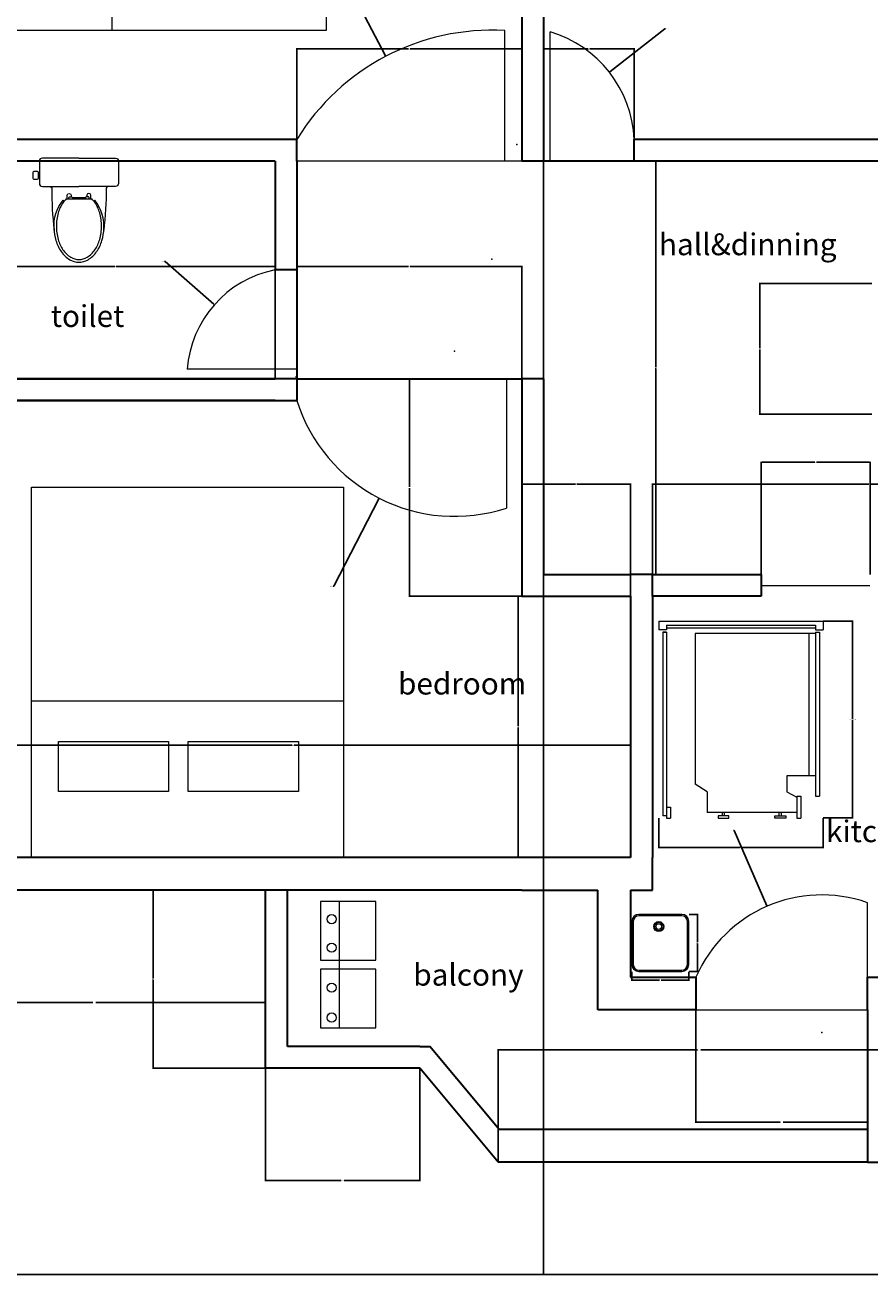
# Model space of a CAD drawing. Units: inches. Extents: x 177 to 785, y -381 to 206.
# Tile 2 of 5: x 296 to 529, y -381 to -37. Entities that reach past the tile are written whole.
import ezdxf

# ---------------------------------------------------------------- set-up
doc = ezdxf.new("R2010")
doc.units = ezdxf.units.IN
doc.header["$MEASUREMENT"] = 0
for name, color, linetype, lineweight in [('A-ANNO-DIMS', 2, 'Continuous', 18), ('A-AREA-IDEN', 7, 'Continuous', 20), ('A-DOOR', 4, 'Continuous', 18), ('A-FLOR-FIXT', 8, 'Continuous', 18), ('A-FURN', 2, 'Continuous', 18), ('A-WALL', 7, 'Continuous', 35), ('equipments', 2, 'Continuous', 18), ('WC-Detail_dwgmodels.com', 9, 'Continuous', 13), ('WC-Outline_dwgmodels.com', 8, 'Continuous', 18)]:
    doc.layers.add(name, color=color, linetype=linetype, lineweight=lineweight)
doc.styles.get("Standard").update_dxf_attribs({"font": 'arial.ttf'})
doc.dimstyles.get("Standard").update_dxf_attribs({"dimtxt": 0.18, "dimasz": 0.18, "dimexe": 0.18, "dimexo": 0.0625, "dimgap": 0.09, "dimtad": 0, "dimtih": 1, "dimtoh": 1, "dimdec": 4, "dimzin": 0, "dimdsep": 46, "dimtxsty": 'Standard', "dimcen": 0.09, "dimadec": 0, "dimazin": 0, "dimtfac": 1, "dimtdec": 4, "dimtofl": 0, "dimtmove": 0, "dimatfit": 3, "dimfxl": 1, "dimtolj": 1, "dimtzin": 0, "dimarcsym": 0})

# ---------------------------------------------------------------- blocks, each defined once
blk = doc.blocks.new('fr1')
at = {"color": 0, "linetype": 'ByBlock'}
for p, q in [((90.8, 438.2), (-210.3, 438.2)), ((-259.7, 390.1), (-259.7, 86.3)), ((-249.7, 390.1), (-249.7, 86.5)), ((90.8, 428.2), (-210.3, 428.2)), ((130.2, 86.5), (130.2, 390.1)), ((140.2, 87.7), (140.2, 390.1)), ((-210.3, 48.2), (90.8, 48.2)), ((-210.3, 38.2), (90.8, 38.2))]:
    blk.add_line(p, q, dxfattribs=at)
for radius in [35, 30, 20]:
    blk.add_circle((-70.8, 353.2), radius)
for centre, radius, start, end in [((-210.3, 388.7), 49.5, 90, 178.38137), ((90.8, 388.7), 49.5, 1.61863, 90), ((-210.3, 388.7), 39.5, 90, 178.38137), ((90.8, 388.7), 39.5, 1.61863, 90), ((-210.3, 87.7), 49.5, 181.61863, 270), ((-210.3, 87.7), 39.5, 181.61863, 270), ((90.8, 87.7), 39.5, 270, 358.38137), ((90.8, 87.7), 49.5, 270, 358.38137)]:
    blk.add_arc(centre, radius, start, end)
at = {"color": 0, "linetype": 'ByBlock', "extrusion": (0, 0, -1)}
blk.add_ellipse((90.8, 87.7), major_axis=(49.5, 0), ratio=1, start_param=0, end_param=0.02825, dxfattribs=at)
blk = doc.blocks.new('dishwasher_smegsta945s')
for p, q in [((0, 90), (75, 90)), ((0, 90), (0, 86)), ((3.5, 86), (0, 86)), ((3.5, 88.1), (71.5, 88.1)), ((3.5, 88.1), (3.5, 86)), ((3.5, 87), (71.5, 87)), ((71.5, 88.1), (71.5, 86)), ((71.5, 86), (75, 86)), ((75, 90), (75, 86)), ((1.7, 85), (1.7, 1)), ((3.5, 85), (1.7, 85)), ((1.7, 85), (3.5, 85)), ((3.5, 85), (3.5, 0)), ((71.5, 84.3), (16.5, 84.3)), ((16.5, 84.3), (16.5, 15.5)), ((68.5, 84.3), (68.5, 19.3)), ((71.5, 85), (71.5, 10)), ((71.5, 85), (73.3, 85)), ((71.5, 85), (73.3, 85)), ((73.3, 85), (73.3, 10)), ((71.5, 19.3), (58.5, 19.3)), ((58.5, 19.3), (58.5, 12)), ((22, 12), (16.5, 15.5)), ((22, 12), (22, 2.5)), ((58.5, 12), (63, 9.5)), ((63, 10), (64.8, 10)), ((63, 10), (63, 0)), ((64.8, 10), (64.8, 0)), ((71.5, 10), (73.3, 10)), ((3.5, 1), (1.7, 1)), ((3.5, 5), (5.3, 5)), ((5.3, 5), (5.3, 0)), ((63, 2.5), (22, 2.5)), ((29, 1), (29, 2.5)), ((30, 1), (30, 2.5)), ((55, 1), (55, 2.5)), ((56, 1), (56, 2.5)), ((63, 0), (64.8, 0)), ((3.5, 0), (5.3, 0))]:
    blk.add_line(p, q)
for points in [[(27, 0), (32, 0), (32, 1), (27, 1)], [(58, 0), (53, 0), (53, 1), (58, 1)]]:
    blk.add_lwpolyline(points, close=True)
blk = doc.blocks.new('BED-DOUBLE')
blk.add_line((58.96, 86.04), (58.96, 0))
for points in [[(0, 86.04), (102.05, 86.04), (102.05, 0), (0, 0)], [(70.1, 73.56), (83.84, 73.56), (83.84, 43.2), (70.1, 43.2)], [(70.1, 37.79), (83.84, 37.79), (83.84, 7.42), (70.1, 7.42)]]:
    blk.add_lwpolyline(points, close=True)
blk = doc.blocks.new('WC-PAN-AND-SEAT')
for points in [[(0, 20.91, -0.279901), (0.43, 20.4, 0.030761), (1.12, 8.8, 16.522544)], [(15.88, 20.91, 0.279901), (15.45, 20.4, -0.030761), (14.76, 8.8, -16.522544)], [(1.72, 9.92, 0.068564), (2.22, 6.28, 0.080689), (3.54, 3.43, 0.107047), (5.7, 1.38, 0.137952), (7.94, 0.75, 0.137952), (10.18, 1.38, 0.107047), (12.34, 3.43, 0.080689), (13.66, 6.28, 0.068564), (14.16, 9.92, 0.068564), (13.66, 13.57, 0.080689), (12.34, 16.41, 0.049741), (11.45, 17.48, 0.137952)], [(4.44, 17.48, 0.049741), (3.54, 16.41, 0.080689), (2.22, 13.57, 0.068564), (1.72, 9.92, 0.068564)], [(1.08, 9.29, -0.186192), (3.55, 17.08), (3.86, 16.84)], [(14.76, 8.8, 0.197511), (12.33, 17.08), (12.02, 16.84)], [(1.07, 9.29, 0.059006), (1.61, 5.99, 0.081908), (3.07, 2.91, 0.106902), (5.45, 0.69, 0.135271), (7.94, 0, 0.135271)], [(1.12, 8.8, -0.010918), (1.08, 9.29)], [(7.94, 0, 0.135271), (10.44, 0.69, 0.106902), (12.81, 2.91, 0.081908), (14.28, 5.99, 0.059006), (14.82, 9.29, 0.070136)]]:
    blk.add_lwpolyline(points, format="xyb")
blk.add_lwpolyline([(4.44, 17.48), (11.45, 17.48)])
blk = doc.blocks.new('*D19')
at = {"layer": 'A-ANNO-DIMS', "color": 0, "lineweight": -2, "transparency": 16777216}
for p, q in [((479.47, -281.84), (481.94, -281.84)), ((481.76, -282.02), (481.76, -289.54)), ((481.76, -297.41), (481.76, -289.9)), ((479.47, -297.59), (481.94, -297.59))]:
    blk.add_line(p, q, dxfattribs=at)
at = {"layer": 'A-ANNO-DIMS', "color": 0, "transparency": 16777216}
for points in [[(481.73, -282.02), (481.79, -282.02), (481.76, -281.84)], [(481.73, -297.41), (481.79, -297.41), (481.76, -297.59)]]:
    blk.add_solid(points, dxfattribs=at)
at = {"layer": 'Defpoints', "color": 0, "transparency": 16777216}
for p in [(479.4, -281.84), (481.76, -281.84), (479.4, -297.59)]:
    blk.add_point(p, dxfattribs=at)
at = {"layer": 'A-ANNO-DIMS', "color": 0, "transparency": 16777216, "insert": (481.76, -289.72), "char_height": 0.18, "attachment_point": 5}
blk.add_mtext('\\A1;SINK 16', dxfattribs=at)
blk = doc.blocks.new('*D20')
at = {"layer": 'A-ANNO-DIMS', "color": 0, "lineweight": -2, "transparency": 16777216}
for p, q in [((463.66, -297.66), (463.66, -300.13)), ((479.4, -297.66), (479.4, -300.13)), ((463.84, -299.95), (471.32, -299.95)), ((479.22, -299.95), (471.74, -299.95))]:
    blk.add_line(p, q, dxfattribs=at)
at = {"layer": 'A-ANNO-DIMS', "color": 0, "transparency": 16777216}
for points in [[(463.84, -299.92), (463.84, -299.98), (463.66, -299.95)], [(479.22, -299.92), (479.22, -299.98), (479.4, -299.95)]]:
    blk.add_solid(points, dxfattribs=at)
at = {"layer": 'Defpoints', "color": 0, "transparency": 16777216}
for p in [(463.66, -297.59), (479.4, -297.59), (479.4, -299.95)]:
    blk.add_point(p, dxfattribs=at)
at = {"layer": 'A-ANNO-DIMS', "color": 0, "transparency": 16777216, "insert": (471.53, -299.95), "char_height": 0.18, "attachment_point": 5}
blk.add_mtext('\\A1;16', dxfattribs=at)
blk = doc.blocks.new('*D21')
at = {"layer": 'A-ANNO-DIMS', "color": 0, "lineweight": -2, "transparency": 16777216}
for p, q in [((516.45, -200.99), (524.71, -200.99)), ((524.53, -201.17), (524.53, -227.94)), ((524.53, -255.08), (524.53, -228.31)), ((516.45, -255.26), (524.71, -255.26))]:
    blk.add_line(p, q, dxfattribs=at)
at = {"layer": 'A-ANNO-DIMS', "color": 0, "transparency": 16777216}
for points in [[(524.5, -201.17), (524.56, -201.17), (524.53, -200.99)], [(524.5, -255.08), (524.56, -255.08), (524.53, -255.26)]]:
    blk.add_solid(points, dxfattribs=at)
at = {"layer": 'Defpoints', "color": 0, "transparency": 16777216}
for p in [(516.39, -200.99), (524.53, -200.99), (516.39, -255.26)]:
    blk.add_point(p, dxfattribs=at)
at = {"layer": 'A-ANNO-DIMS', "color": 0, "transparency": 16777216, "insert": (524.53, -228.12), "char_height": 0.18, "attachment_point": 5}
blk.add_mtext('\\A1;DISHWASHER 54', dxfattribs=at)
blk = doc.blocks.new('*D22')
at = {"layer": 'A-ANNO-DIMS', "color": 0, "lineweight": -2, "transparency": 16777216}
for p, q in [((471.16, -255.32), (471.16, -263.58)), ((516.39, -255.32), (516.39, -263.58)), ((471.34, -263.4), (493.55, -263.4)), ((516.21, -263.4), (494, -263.4))]:
    blk.add_line(p, q, dxfattribs=at)
at = {"layer": 'A-ANNO-DIMS', "color": 0, "transparency": 16777216}
for points in [[(471.34, -263.37), (471.34, -263.43), (471.16, -263.4)], [(516.21, -263.37), (516.21, -263.43), (516.39, -263.4)]]:
    blk.add_solid(points, dxfattribs=at)
at = {"layer": 'Defpoints', "color": 0, "transparency": 16777216}
for p in [(471.16, -255.26), (516.39, -255.26), (516.39, -263.4)]:
    blk.add_point(p, dxfattribs=at)
at = {"layer": 'A-ANNO-DIMS', "color": 0, "transparency": 16777216, "insert": (493.77, -263.4), "char_height": 0.18, "attachment_point": 5}
blk.add_mtext('\\A1;45', dxfattribs=at)
blk = doc.blocks.new('*D23')
at = {"layer": 'A-ANNO-DIMS', "color": 0, "lineweight": -2, "transparency": 16777216}
for p, q in [((754.33, -257.2), (754.33, -381.27)), ((202.33, -275.2), (202.33, -381.27)), ((202.51, -381.09), (478.04, -381.09)), ((754.15, -381.09), (478.62, -381.09))]:
    blk.add_line(p, q, dxfattribs=at)
at = {"layer": 'A-ANNO-DIMS', "color": 0, "transparency": 16777216}
for points in [[(202.51, -381.06), (202.51, -381.12), (202.33, -381.09)], [(754.15, -381.06), (754.15, -381.12), (754.33, -381.09)]]:
    blk.add_solid(points, dxfattribs=at)
at = {"layer": 'Defpoints', "color": 0, "transparency": 16777216}
for p in [(754.33, -257.14), (202.33, -275.14), (754.33, -381.09)]:
    blk.add_point(p, dxfattribs=at)
at = {"layer": 'A-ANNO-DIMS', "color": 0, "transparency": 16777216, "insert": (478.33, -381.09), "char_height": 0.18, "attachment_point": 5}
blk.add_mtext('\\A1;552', dxfattribs=at)
blk = doc.blocks.new('*D33')
at = {"layer": 'A-ANNO-DIMS', "color": 0, "lineweight": -2, "transparency": 16777216}
for p, q in [((607.33, -68.2), (607.33, -381.27)), ((439.33, -74.2), (439.33, -381.27)), ((439.51, -381.09), (523.05, -381.09)), ((607.15, -381.09), (523.61, -381.09))]:
    blk.add_line(p, q, dxfattribs=at)
at = {"layer": 'A-ANNO-DIMS', "color": 0, "transparency": 16777216}
for points in [[(439.51, -381.06), (439.51, -381.12), (439.33, -381.09)], [(607.15, -381.06), (607.15, -381.12), (607.33, -381.09)]]:
    blk.add_solid(points, dxfattribs=at)
at = {"layer": 'Defpoints', "color": 0, "transparency": 16777216}
for p in [(607.33, -68.14), (439.33, -74.14), (607.33, -381.09)]:
    blk.add_point(p, dxfattribs=at)
at = {"layer": 'A-ANNO-DIMS', "color": 0, "transparency": 16777216, "insert": (523.33, -381.09), "char_height": 0.18, "attachment_point": 5}
blk.add_mtext('\\A1;168', dxfattribs=at)
blk = doc.blocks.new('*D41')
at = {"layer": 'A-ANNO-DIMS', "color": 0, "lineweight": -2, "transparency": 16777216}
for p, q in [((277.33, -134.08), (277.33, -103.01)), ((277.51, -103.19), (321.11, -103.19)), ((365.15, -103.19), (321.55, -103.19)), ((365.33, -134.08), (365.33, -103.01))]:
    blk.add_line(p, q, dxfattribs=at)
at = {"layer": 'A-ANNO-DIMS', "color": 0, "transparency": 16777216}
for points in [[(277.51, -103.16), (277.51, -103.22), (277.33, -103.19)], [(365.15, -103.16), (365.15, -103.22), (365.33, -103.19)]]:
    blk.add_solid(points, dxfattribs=at)
at = {"layer": 'Defpoints', "color": 0, "transparency": 16777216}
for p in [(365.33, -103.19), (277.33, -134.14), (365.33, -134.14)]:
    blk.add_point(p, dxfattribs=at)
at = {"layer": 'A-ANNO-DIMS', "color": 0, "transparency": 16777216, "insert": (321.33, -103.19), "char_height": 0.18, "attachment_point": 5}
blk.add_mtext('\\A1;88', dxfattribs=at)
blk = doc.blocks.new('*D45')
at = {"layer": 'A-ANNO-DIMS', "color": 0, "lineweight": -2, "transparency": 16777216}
for p, q in [((277.33, -266.08), (277.33, -235.01)), ((277.51, -235.19), (370.05, -235.19)), ((463.15, -235.19), (370.61, -235.19)), ((463.33, -266.08), (463.33, -235.01))]:
    blk.add_line(p, q, dxfattribs=at)
at = {"layer": 'A-ANNO-DIMS', "color": 0, "transparency": 16777216}
for points in [[(277.51, -235.16), (277.51, -235.22), (277.33, -235.19)], [(463.15, -235.16), (463.15, -235.22), (463.33, -235.19)]]:
    blk.add_solid(points, dxfattribs=at)
at = {"layer": 'Defpoints', "color": 0, "transparency": 16777216}
for p in [(463.33, -235.19), (277.33, -266.14), (463.33, -266.14)]:
    blk.add_point(p, dxfattribs=at)
at = {"layer": 'A-ANNO-DIMS', "color": 0, "transparency": 16777216, "insert": (370.33, -235.19), "char_height": 0.18, "attachment_point": 5}
blk.add_mtext('\\A1;186', dxfattribs=at)
blk = doc.blocks.new('*D46')
at = {"layer": 'A-ANNO-DIMS', "color": 0, "lineweight": -2, "transparency": 16777216}
for p, q in [((433.27, -134.14), (402.2, -134.14)), ((402.38, -134.32), (402.38, -163.96)), ((402.38, -193.96), (402.38, -164.32)), ((433.27, -194.14), (402.2, -194.14))]:
    blk.add_line(p, q, dxfattribs=at)
at = {"layer": 'A-ANNO-DIMS', "color": 0, "transparency": 16777216}
for points in [[(402.35, -134.32), (402.41, -134.32), (402.38, -134.14)], [(402.35, -193.96), (402.41, -193.96), (402.38, -194.14)]]:
    blk.add_solid(points, dxfattribs=at)
at = {"layer": 'Defpoints', "color": 0, "transparency": 16777216}
for p in [(402.38, -134.14), (433.33, -134.14), (433.33, -194.14)]:
    blk.add_point(p, dxfattribs=at)
at = {"layer": 'A-ANNO-DIMS', "color": 0, "transparency": 16777216, "insert": (402.38, -164.14), "char_height": 0.18, "attachment_point": 5}
blk.add_mtext('\\A1;60', dxfattribs=at)
blk = doc.blocks.new('*D47')
at = {"layer": 'A-ANNO-DIMS', "color": 0, "lineweight": -2, "transparency": 16777216}
for p, q in [((463.27, -194.14), (432.2, -194.14)), ((432.38, -194.32), (432.38, -229.96)), ((432.38, -265.96), (432.38, -230.32)), ((463.27, -266.14), (432.2, -266.14))]:
    blk.add_line(p, q, dxfattribs=at)
at = {"layer": 'A-ANNO-DIMS', "color": 0, "transparency": 16777216}
for points in [[(432.35, -194.32), (432.41, -194.32), (432.38, -194.14)], [(432.35, -265.96), (432.41, -265.96), (432.38, -266.14)]]:
    blk.add_solid(points, dxfattribs=at)
at = {"layer": 'Defpoints', "color": 0, "transparency": 16777216}
for p in [(432.38, -194.14), (463.33, -194.14), (463.33, -266.14)]:
    blk.add_point(p, dxfattribs=at)
at = {"layer": 'A-ANNO-DIMS', "color": 0, "transparency": 16777216, "insert": (432.38, -230.14), "char_height": 0.18, "attachment_point": 5}
blk.add_mtext('\\A1;72', dxfattribs=at)
blk = doc.blocks.new('*D48')
at = {"layer": 'A-ANNO-DIMS', "color": 0, "lineweight": -2, "transparency": 16777216}
for p, q in [((433.33, -194.08), (433.33, -163.01)), ((433.51, -163.19), (448.11, -163.19)), ((463.15, -163.19), (448.55, -163.19)), ((463.33, -194.08), (463.33, -163.01))]:
    blk.add_line(p, q, dxfattribs=at)
at = {"layer": 'A-ANNO-DIMS', "color": 0, "transparency": 16777216}
for points in [[(433.51, -163.16), (433.51, -163.22), (433.33, -163.19)], [(463.15, -163.16), (463.15, -163.22), (463.33, -163.19)]]:
    blk.add_solid(points, dxfattribs=at)
at = {"layer": 'Defpoints', "color": 0, "transparency": 16777216}
for p in [(463.33, -163.19), (433.33, -194.14), (463.33, -194.14)]:
    blk.add_point(p, dxfattribs=at)
at = {"layer": 'A-ANNO-DIMS', "color": 0, "transparency": 16777216, "insert": (448.33, -163.19), "char_height": 0.18, "attachment_point": 5}
blk.add_mtext('\\A1;30', dxfattribs=at)
blk = doc.blocks.new('*D49')
at = {"layer": 'A-ANNO-DIMS', "color": 0, "lineweight": -2, "transparency": 16777216}
for p, q in [((469.33, -194.08), (469.33, -163.01)), ((469.51, -163.19), (529.05, -163.19)), ((589.15, -163.19), (529.61, -163.19)), ((589.33, -194.08), (589.33, -163.01))]:
    blk.add_line(p, q, dxfattribs=at)
at = {"layer": 'A-ANNO-DIMS', "color": 0, "transparency": 16777216}
for points in [[(469.51, -163.16), (469.51, -163.22), (469.33, -163.19)], [(589.15, -163.16), (589.15, -163.22), (589.33, -163.19)]]:
    blk.add_solid(points, dxfattribs=at)
at = {"layer": 'Defpoints', "color": 0, "transparency": 16777216}
for p in [(589.33, -163.19), (469.33, -194.14), (589.33, -194.14)]:
    blk.add_point(p, dxfattribs=at)
at = {"layer": 'A-ANNO-DIMS', "color": 0, "transparency": 16777216, "insert": (529.33, -163.19), "char_height": 0.18, "attachment_point": 5}
blk.add_mtext('\\A1;120', dxfattribs=at)
blk = doc.blocks.new('*D54')
at = {"layer": 'A-ANNO-DIMS', "color": 0, "lineweight": -2, "transparency": 16777216}
for p, q in [((439.39, -74.14), (470.46, -74.14)), ((470.28, -74.32), (470.28, -130.96)), ((470.28, -187.96), (470.28, -131.32)), ((439.39, -188.14), (470.46, -188.14))]:
    blk.add_line(p, q, dxfattribs=at)
at = {"layer": 'A-ANNO-DIMS', "color": 0, "transparency": 16777216}
for points in [[(470.25, -74.32), (470.31, -74.32), (470.28, -74.14)], [(470.25, -187.96), (470.31, -187.96), (470.28, -188.14)]]:
    blk.add_solid(points, dxfattribs=at)
at = {"layer": 'Defpoints', "color": 0, "transparency": 16777216}
for p in [(439.33, -74.14), (439.33, -188.14), (470.28, -188.14)]:
    blk.add_point(p, dxfattribs=at)
at = {"layer": 'A-ANNO-DIMS', "color": 0, "transparency": 16777216, "insert": (470.28, -131.14), "char_height": 0.18, "attachment_point": 5}
blk.add_mtext('\\A1;114', dxfattribs=at)
blk = doc.blocks.new('*D56')
at = {"layer": 'A-ANNO-DIMS', "color": 0, "lineweight": -2, "transparency": 16777216}
for p, q in [((362.64, -275.14), (331.57, -275.14)), ((331.75, -275.32), (331.75, -299.53)), ((331.75, -324.1), (331.75, -299.89)), ((362.64, -324.28), (331.57, -324.28))]:
    blk.add_line(p, q, dxfattribs=at)
at = {"layer": 'A-ANNO-DIMS', "color": 0, "transparency": 16777216}
for points in [[(331.72, -275.32), (331.78, -275.32), (331.75, -275.14)], [(331.72, -324.1), (331.78, -324.1), (331.75, -324.28)]]:
    blk.add_solid(points, dxfattribs=at)
at = {"layer": 'Defpoints', "color": 0, "transparency": 16777216}
for p in [(331.75, -275.14), (362.7, -275.14), (362.7, -324.28)]:
    blk.add_point(p, dxfattribs=at)
at = {"layer": 'A-ANNO-DIMS', "color": 0, "transparency": 16777216, "insert": (331.75, -299.71), "char_height": 0.18, "attachment_point": 5}
blk.add_mtext('\\A1;49.14', dxfattribs=at)
blk = doc.blocks.new('*D57')
at = {"layer": 'A-ANNO-DIMS', "color": 0, "lineweight": -2, "transparency": 16777216}
for p, q in [((426.79, -350.08), (426.79, -319.01)), ((426.97, -319.19), (481.74, -319.19)), ((537.43, -319.19), (482.65, -319.19)), ((537.61, -350.08), (537.61, -319.01))]:
    blk.add_line(p, q, dxfattribs=at)
at = {"layer": 'A-ANNO-DIMS', "color": 0, "transparency": 16777216}
for points in [[(426.97, -319.16), (426.97, -319.22), (426.79, -319.19)], [(537.43, -319.16), (537.43, -319.22), (537.61, -319.19)]]:
    blk.add_solid(points, dxfattribs=at)
at = {"layer": 'Defpoints', "color": 0, "transparency": 16777216}
for p in [(537.61, -319.19), (426.79, -350.14), (537.61, -350.14)]:
    blk.add_point(p, dxfattribs=at)
at = {"layer": 'A-ANNO-DIMS', "color": 0, "transparency": 16777216, "insert": (482.2, -319.19), "char_height": 0.18, "attachment_point": 5}
blk.add_mtext('\\A1;110.82', dxfattribs=at)
blk = doc.blocks.new('*D58')
at = {"layer": 'A-ANNO-DIMS', "color": 0, "lineweight": -2, "transparency": 16777216}
for p, q in [((371.33, -74.08), (371.33, -43.01)), ((371.51, -43.19), (402.11, -43.19)), ((433.15, -43.19), (402.55, -43.19)), ((433.33, -74.08), (433.33, -43.01))]:
    blk.add_line(p, q, dxfattribs=at)
at = {"layer": 'A-ANNO-DIMS', "color": 0, "transparency": 16777216}
for points in [[(371.51, -43.16), (371.51, -43.22), (371.33, -43.19)], [(433.15, -43.16), (433.15, -43.22), (433.33, -43.19)]]:
    blk.add_solid(points, dxfattribs=at)
at = {"layer": 'Defpoints', "color": 0, "transparency": 16777216}
for p in [(433.33, -43.19), (371.33, -74.14), (433.33, -74.14)]:
    blk.add_point(p, dxfattribs=at)
at = {"layer": 'A-ANNO-DIMS', "color": 0, "transparency": 16777216, "insert": (402.33, -43.19), "char_height": 0.18, "attachment_point": 5}
blk.add_mtext('\\A1;62', dxfattribs=at)
blk = doc.blocks.new('*D59')
at = {"layer": 'A-ANNO-DIMS', "color": 0, "lineweight": -2, "transparency": 16777216}
for p, q in [((439.33, -74.08), (439.33, -43.01)), ((439.51, -43.19), (451.61, -43.19)), ((464.15, -43.19), (452.05, -43.19)), ((464.33, -74.08), (464.33, -43.01))]:
    blk.add_line(p, q, dxfattribs=at)
at = {"layer": 'A-ANNO-DIMS', "color": 0, "transparency": 16777216}
for points in [[(439.51, -43.16), (439.51, -43.22), (439.33, -43.19)], [(464.15, -43.16), (464.15, -43.22), (464.33, -43.19)]]:
    blk.add_solid(points, dxfattribs=at)
at = {"layer": 'Defpoints', "color": 0, "transparency": 16777216}
for p in [(464.33, -43.19), (439.33, -74.14), (464.33, -74.14)]:
    blk.add_point(p, dxfattribs=at)
at = {"layer": 'A-ANNO-DIMS', "color": 0, "transparency": 16777216, "insert": (451.83, -43.19), "char_height": 0.18, "attachment_point": 5}
blk.add_mtext('\\A1;25', dxfattribs=at)
blk = doc.blocks.new('*D60')
at = {"layer": 'A-ANNO-DIMS', "color": 0, "lineweight": -2, "transparency": 16777216}
for p, q in [((371.33, -134.08), (371.33, -103.01)), ((371.51, -103.19), (402.11, -103.19)), ((433.15, -103.19), (402.55, -103.19)), ((433.33, -134.08), (433.33, -103.01))]:
    blk.add_line(p, q, dxfattribs=at)
at = {"layer": 'A-ANNO-DIMS', "color": 0, "transparency": 16777216}
for points in [[(371.51, -103.16), (371.51, -103.22), (371.33, -103.19)], [(433.15, -103.16), (433.15, -103.22), (433.33, -103.19)]]:
    blk.add_solid(points, dxfattribs=at)
at = {"layer": 'Defpoints', "color": 0, "transparency": 16777216}
for p in [(433.33, -103.19), (371.33, -134.14), (433.33, -134.14)]:
    blk.add_point(p, dxfattribs=at)
at = {"layer": 'A-ANNO-DIMS', "color": 0, "transparency": 16777216, "insert": (402.33, -103.19), "char_height": 0.18, "attachment_point": 5}
blk.add_mtext('\\A1;62', dxfattribs=at)
blk = doc.blocks.new('*D61')
at = {"layer": 'A-ANNO-DIMS', "color": 0, "lineweight": -2, "transparency": 16777216}
for p, q in [((499.33, -188.08), (499.33, -157.01)), ((499.51, -157.19), (514.11, -157.19)), ((529.15, -157.19), (514.55, -157.19)), ((529.33, -188.08), (529.33, -157.01))]:
    blk.add_line(p, q, dxfattribs=at)
at = {"layer": 'A-ANNO-DIMS', "color": 0, "transparency": 16777216}
for points in [[(499.51, -157.16), (499.51, -157.22), (499.33, -157.19)], [(529.15, -157.16), (529.15, -157.22), (529.33, -157.19)]]:
    blk.add_solid(points, dxfattribs=at)
at = {"layer": 'Defpoints', "color": 0, "transparency": 16777216}
for p in [(529.33, -157.19), (499.33, -188.14), (529.33, -188.14)]:
    blk.add_point(p, dxfattribs=at)
at = {"layer": 'A-ANNO-DIMS', "color": 0, "transparency": 16777216, "insert": (514.33, -157.19), "char_height": 0.18, "attachment_point": 5}
blk.add_mtext('\\A1;30', dxfattribs=at)
blk = doc.blocks.new('*D62')
at = {"layer": 'A-ANNO-DIMS', "color": 0, "lineweight": -2, "transparency": 16777216}
for p, q in [((481.33, -308.2), (481.33, -339.27)), ((528.61, -308.2), (528.61, -339.27)), ((481.51, -339.09), (504.57, -339.09)), ((528.43, -339.09), (505.37, -339.09))]:
    blk.add_line(p, q, dxfattribs=at)
at = {"layer": 'A-ANNO-DIMS', "color": 0, "transparency": 16777216}
for points in [[(481.51, -339.06), (481.51, -339.12), (481.33, -339.09)], [(528.43, -339.06), (528.43, -339.12), (528.61, -339.09)]]:
    blk.add_solid(points, dxfattribs=at)
at = {"layer": 'Defpoints', "color": 0, "transparency": 16777216}
for p in [(481.33, -308.14), (528.61, -308.14), (481.33, -339.09)]:
    blk.add_point(p, dxfattribs=at)
at = {"layer": 'A-ANNO-DIMS', "color": 0, "transparency": 16777216, "insert": (504.97, -339.09), "char_height": 0.18, "attachment_point": 5}
blk.add_mtext('\\A1;47.28', dxfattribs=at)
blk = doc.blocks.new('*D65')
at = {"layer": 'A-ANNO-DIMS', "color": 0, "lineweight": -2, "transparency": 16777216}
for p, q in [((268.33, -275.2), (268.33, -306.27)), ((362.7, -275.2), (362.7, -306.27)), ((268.51, -306.09), (315.12, -306.09)), ((362.52, -306.09), (315.91, -306.09))]:
    blk.add_line(p, q, dxfattribs=at)
at = {"layer": 'A-ANNO-DIMS', "color": 0, "transparency": 16777216}
for points in [[(268.51, -306.06), (268.51, -306.12), (268.33, -306.09)], [(362.52, -306.06), (362.52, -306.12), (362.7, -306.09)]]:
    blk.add_solid(points, dxfattribs=at)
at = {"layer": 'Defpoints', "color": 0, "transparency": 16777216}
for p in [(268.33, -275.14), (362.7, -275.14), (268.33, -306.09)]:
    blk.add_point(p, dxfattribs=at)
at = {"layer": 'A-ANNO-DIMS', "color": 0, "transparency": 16777216, "insert": (315.51, -306.09), "char_height": 0.18, "attachment_point": 5}
blk.add_mtext('\\A1;94.37', dxfattribs=at)
blk = doc.blocks.new('*D67')
at = {"layer": 'A-ANNO-DIMS', "color": 0, "lineweight": -2, "transparency": 16777216}
for p, q in [((529.87, -107.85), (498.8, -107.85)), ((498.98, -108.03), (498.98, -125.71)), ((498.98, -143.76), (498.98, -126.07)), ((529.87, -143.94), (498.8, -143.94))]:
    blk.add_line(p, q, dxfattribs=at)
at = {"layer": 'A-ANNO-DIMS', "color": 0, "transparency": 16777216}
for points in [[(498.95, -108.03), (499.01, -108.03), (498.98, -107.85)], [(498.95, -143.76), (499.01, -143.76), (498.98, -143.94)]]:
    blk.add_solid(points, dxfattribs=at)
at = {"layer": 'Defpoints', "color": 0, "transparency": 16777216}
for p in [(498.98, -107.85), (529.93, -107.85), (529.93, -143.94)]:
    blk.add_point(p, dxfattribs=at)
at = {"layer": 'A-ANNO-DIMS', "color": 0, "transparency": 16777216, "insert": (498.98, -125.89), "char_height": 0.18, "attachment_point": 5}
blk.add_mtext('\\A1;36.09', dxfattribs=at)
blk = doc.blocks.new('*D73')
at = {"layer": 'A-ANNO-DIMS', "color": 0, "lineweight": -2, "transparency": 16777216}
for p, q in [((362.7, -324.34), (362.7, -355.41)), ((405.22, -324.34), (405.22, -355.41)), ((362.88, -355.23), (383.56, -355.23)), ((405.04, -355.23), (384.36, -355.23))]:
    blk.add_line(p, q, dxfattribs=at)
at = {"layer": 'A-ANNO-DIMS', "color": 0, "transparency": 16777216}
for points in [[(362.88, -355.2), (362.88, -355.26), (362.7, -355.23)], [(405.04, -355.2), (405.04, -355.26), (405.22, -355.23)]]:
    blk.add_solid(points, dxfattribs=at)
at = {"layer": 'Defpoints', "color": 0, "transparency": 16777216}
for p in [(362.7, -324.28), (405.22, -324.28), (362.7, -355.23)]:
    blk.add_point(p, dxfattribs=at)
at = {"layer": 'A-ANNO-DIMS', "color": 0, "transparency": 16777216, "insert": (383.96, -355.23), "char_height": 0.18, "attachment_point": 5}
blk.add_mtext('\\A1;42.52', dxfattribs=at)
blk = doc.blocks.new('*D74')
at = {"layer": 'A-ANNO-DIMS', "color": 0, "lineweight": -2, "transparency": 16777216}
for p, q in [((378.1, -11.7), (378.28, -11.7)), ((378.28, -11.7), (395.76, -45.08)), ((425.02, -101.14), (425.2, -101.14)), ((425.11, -101.23), (425.11, -101.05))]:
    blk.add_line(p, q, dxfattribs=at)
at = {"layer": 'A-ANNO-DIMS', "color": 0, "transparency": 16777216}
blk.add_solid([(395.78, -45.07), (395.73, -45.1), (395.84, -45.24)], dxfattribs=at)
at = {"layer": 'Defpoints', "color": 0, "transparency": 16777216}
for p in [(395.84, -45.24), (425.11, -101.14)]:
    blk.add_point(p, dxfattribs=at)
at = {"layer": 'A-ANNO-DIMS', "color": 0, "transparency": 16777216, "insert": (377.7, -11.7), "char_height": 0.18, "attachment_point": 5}
blk.add_mtext('\\A1;R63.1', dxfattribs=at)
blk = doc.blocks.new('*D76')
at = {"layer": 'A-ANNO-DIMS', "color": 0, "lineweight": -2, "transparency": 16777216}
for p, q in [((414.7, -126.55), (414.88, -126.55)), ((414.79, -126.64), (414.79, -126.46)), ((381.51, -191.37), (393.91, -167.22)), ((381.33, -191.37), (381.51, -191.37))]:
    blk.add_line(p, q, dxfattribs=at)
at = {"layer": 'A-ANNO-DIMS', "color": 0, "transparency": 16777216}
blk.add_solid([(393.88, -167.21), (393.94, -167.23), (393.99, -167.06)], dxfattribs=at)
at = {"layer": 'Defpoints', "color": 0, "transparency": 16777216}
for p in [(414.79, -126.55), (393.99, -167.06)]:
    blk.add_point(p, dxfattribs=at)
at = {"layer": 'A-ANNO-DIMS', "color": 0, "transparency": 16777216, "insert": (380.85, -191.37), "char_height": 0.18, "attachment_point": 5}
blk.add_mtext('\\A1;R45.54', dxfattribs=at)
blk = doc.blocks.new('*D77')
at = {"layer": 'A-ANNO-DIMS', "color": 0, "lineweight": -2, "transparency": 16777216}
for p, q in [((491.71, -258.74), (491.89, -258.74)), ((491.89, -258.74), (500.87, -279.44)), ((515.95, -314.38), (516.13, -314.38)), ((516.04, -314.47), (516.04, -314.29))]:
    blk.add_line(p, q, dxfattribs=at)
at = {"layer": 'A-ANNO-DIMS', "color": 0, "transparency": 16777216}
blk.add_solid([(500.9, -279.43), (500.85, -279.45), (500.94, -279.61)], dxfattribs=at)
at = {"layer": 'Defpoints', "color": 0, "transparency": 16777216}
for p in [(500.94, -279.61), (516.04, -314.38)]:
    blk.add_point(p, dxfattribs=at)
at = {"layer": 'A-ANNO-DIMS', "color": 0, "transparency": 16777216, "insert": (491.25, -258.74), "char_height": 0.18, "attachment_point": 5}
blk.add_mtext('\\A1;R37.91', dxfattribs=at)
blk = doc.blocks.new('*D78')
at = {"layer": 'A-ANNO-DIMS', "color": 0, "lineweight": -2, "transparency": 16777216}
for p, q in [((472.76, -37.63), (457.61, -49.5)), ((472.94, -37.63), (472.76, -37.63)), ((431.9, -69.57), (432.08, -69.57)), ((431.99, -69.66), (431.99, -69.48))]:
    blk.add_line(p, q, dxfattribs=at)
at = {"layer": 'A-ANNO-DIMS', "color": 0, "transparency": 16777216}
blk.add_solid([(457.59, -49.47), (457.63, -49.52), (457.47, -49.61)], dxfattribs=at)
at = {"layer": 'Defpoints', "color": 0, "transparency": 16777216}
for p in [(457.47, -49.61), (431.99, -69.57)]:
    blk.add_point(p, dxfattribs=at)
at = {"layer": 'A-ANNO-DIMS', "color": 0, "transparency": 16777216, "insert": (473.42, -37.63), "char_height": 0.18, "attachment_point": 5}
blk.add_mtext('\\A1;R32.37', dxfattribs=at)
blk = doc.blocks.new('*D79')
at = {"layer": 'A-ANNO-DIMS', "color": 0, "lineweight": -2, "transparency": 16777216}
for p, q in [((334.87, -101.79), (335.05, -101.79)), ((335.05, -101.79), (348.44, -113.62)), ((371.03, -133.66), (371.21, -133.66)), ((371.12, -133.75), (371.12, -133.57))]:
    blk.add_line(p, q, dxfattribs=at)
at = {"layer": 'A-ANNO-DIMS', "color": 0, "transparency": 16777216}
blk.add_solid([(348.46, -113.6), (348.42, -113.64), (348.57, -113.74)], dxfattribs=at)
at = {"layer": 'Defpoints', "color": 0, "transparency": 16777216}
for p in [(348.57, -113.74), (371.12, -133.66)]:
    blk.add_point(p, dxfattribs=at)
at = {"layer": 'A-ANNO-DIMS', "color": 0, "transparency": 16777216, "insert": (334.32, -101.79), "char_height": 0.18, "attachment_point": 5}
blk.add_mtext('\\A1;R30.087', dxfattribs=at)

msp = doc.modelspace()

# ---------------------------------------------------------------- linework, layer by layer
at = {"layer": 'A-DOOR'}
for p, q in [((428.6202, -74.1401), (428.6202, -38.1401)), ((441.1154, -74.1401), (441.1154, -38.5162)), ((433.3284, -74.1401), (371.3284, -74.1401)), ((371.3284, -131.5482), (341.106, -131.5482)), ((429.0779, -134.1401), (429.0779, -169.7877)), ((499.3284, -191.1401), (529.3284, -191.1401)), ((528.6096, -308.1401), (528.6096, -278.6179)), ((481.3284, -308.1401), (528.6096, -308.1401))]:
    msp.add_line(p, q, dxfattribs=at)
for centre, radius, start, end in [((425.1088, -101.1401), 63.0978, 86.809847, 148.466446), ((431.9914, -69.5736), 32.3699, 2.538191, 73.628307), ((371.1181, -133.6644), 30.0867, 101.094926, 175.966591), ((414.7917, -126.5473), 45.5393, 197.366629, 288.283034), ((516.0372, -314.379), 37.9068, 70.629909, 156.296067)]:
    msp.add_arc(centre, radius, start, end, dxfattribs=at)
at = {"layer": 'A-WALL'}
for p, q in [((433.3284, 93.8599), (433.3284, -38.1401)), ((439.3284, 93.8599), (439.3284, -38.1401)), ((433.3284, -38.1401), (433.3284, -74.1401)), ((439.3284, -38.1401), (439.3284, -74.1401)), ((371.3284, -68.1401), (277.3284, -68.1401)), ((371.3284, -74.1401), (371.3284, -68.1401)), ((495.3305, -68.1401), (464.3295, -68.1401)), ((464.3295, -74.1401), (464.3295, -68.1401)), ((607.3284, -68.1401), (495.3305, -68.1401)), ((365.3284, -74.1401), (277.3284, -74.1401)), ((365.3284, -74.1401), (365.3284, -104.1401)), ((371.3284, -74.1401), (371.3284, -134.1401)), ((495.3305, -74.1401), (433.3284, -74.1401)), ((613.3284, -74.1401), (495.3305, -74.1401)), ((371.3284, -104.1401), (365.3284, -104.1401)), ((365.3284, -134.1401), (277.3284, -134.1401)), ((277.3284, -134.1401), (365.3284, -134.1401)), ((371.3284, -134.1401), (365.3284, -134.1401)), ((371.3284, -134.1401), (433.3284, -134.1401)), ((371.3284, -134.1401), (371.3284, -140.1401)), ((433.3284, -134.1401), (433.3284, -194.1401)), ((433.3284, -134.1401), (433.3284, -194.1401)), ((439.3284, -134.1401), (433.3284, -134.1401)), ((439.3284, -134.1401), (439.3284, -188.1401)), ((365.3284, -140.1401), (277.3284, -140.1401)), ((277.3284, -140.1401), (371.3284, -140.1401)), ((365.3284, -140.1401), (371.3284, -140.1401)), ((439.3284, -188.1401), (463.3284, -188.1401)), ((469.3284, -188.1401), (463.3284, -188.1401)), ((469.3284, -194.1401), (469.3284, -188.1401)), ((469.3284, -188.1401), (499.3284, -188.1401)), ((499.3284, -188.1401), (499.3284, -194.1401)), ((433.3284, -194.1401), (463.3284, -194.1401)), ((463.3284, -194.1401), (463.3284, -266.1401)), ((469.3284, -194.1401), (469.3284, -266.1401)), ((499.3284, -194.1401), (469.3284, -194.1401)), ((433.3284, -266.1401), (277.3284, -266.1401)), ((463.3284, -266.1401), (433.3284, -266.1401)), ((469.3284, -275.1401), (469.3284, -266.1401)), ((433.3284, -275.1401), (277.3284, -275.1401)), ((362.6997, -324.2759), (362.6997, -275.1401)), ((368.6997, -318.2759), (368.6997, -275.1401)), ((433.3284, -275.1401), (454.3284, -275.1401)), ((454.3284, -308.1401), (454.3284, -275.1401)), ((463.3284, -275.1401), (463.3284, -299.1401)), ((463.3284, -275.1401), (469.3284, -275.1401)), ((463.3284, -299.1401), (481.3284, -299.1401)), ((481.3284, -299.1401), (481.3284, -308.1401)), ((528.6096, -308.1401), (528.6096, -299.1401)), ((528.6096, -299.1401), (589.3284, -299.1401)), ((463.3284, -308.1401), (454.3284, -308.1401)), ((481.3284, -308.1401), (463.3284, -308.1401)), ((528.6096, -308.1401), (528.6096, -350.1401)), ((405.218, -318.2759), (368.6997, -318.2759)), ((405.218, -318.2759), (408.0031, -318.2759)), ((409.8259, -320.4331), (408.0031, -318.2759)), ((427.0945, -341.1401), (409.8259, -320.4331)), ((405.218, -324.2759), (362.6997, -324.2759)), ((426.7874, -350.1401), (405.218, -324.2759)), ((528.6096, -341.1401), (427.0945, -341.1401)), ((528.6096, -350.1401), (426.7874, -350.1401)), ((528.6096, -350.1401), (537.6096, -350.1401))]:
    msp.add_line(p, q, dxfattribs=at)
at = {"layer": 'equipments'}
for p, q in [((383.0801, -294.4898), (383.0801, -278.2823)), ((383.0801, -296.921), (383.0801, -294.4898)), ((383.0801, -313.1284), (383.0801, -296.921))]:
    msp.add_line(p, q, dxfattribs=at)
for points in [[(377.8734, -294.4898), (393.0791, -294.4898), (393.0791, -278.2823), (377.8734, -278.2823)], [(377.8734, -313.1284), (393.0791, -313.1284), (393.0791, -296.921), (377.8734, -296.921)]]:
    msp.add_lwpolyline(points, close=True, dxfattribs=at)
for centre in [(380.9234, -283.1532), (380.9234, -291.0137), (380.9234, -302.0437), (380.9234, -310.2844)]:
    msp.add_circle(centre, 1.2687, dxfattribs=at)
at = {"layer": 'WC-Detail_dwgmodels.com'}
for points in [[(300.1079, -78.6677), (300.1079, -77.4078, 0.41421356)], [(307.982, -84.5338), (307.982, -83.5102, -0.78819772), (309.0843, -83.5102), (309.0843, -83.9826)], [(308.4544, -84.5338), (308.4544, -84.1795, -0.41421356), (308.6512, -83.9826), (309.2418, -83.9826, -0.41421356), (309.4386, -84.1795), (309.4386, -84.5338)], [(314.0449, -84.5338), (314.0449, -84.1795, 0.41421356), (313.8481, -83.9826), (313.2575, -83.9826, 0.41421356), (313.0607, -84.1795), (313.0607, -84.5338)], [(314.5174, -84.5338), (314.5174, -83.5102, 0.78819772), (313.415, -83.5102), (313.415, -83.9826)]]:
    msp.add_lwpolyline(points, format="xyb", dxfattribs=at)
msp.add_lwpolyline([(309.4386, -84.1401), (313.0607, -84.1401)], dxfattribs=at)
at = {"layer": 'WC-Outline_dwgmodels.com'}
for points in [[(311.2497, -73.3133), (301.1709, -73.3133, 0.41421356), (300.3442, -74.1401), (300.3442, -77.4078, 0.41421356)], [(311.2497, -73.3133), (321.3284, -73.3133, -0.41421356), (322.1552, -74.1401), (322.1552, -80.2818, -0.41421356), (321.3284, -81.1086), (319.1914, -81.1086)], [(300.1079, -77.4078), (300.1079, -77.2503, 0.41421356), (299.8323, -76.9747), (298.8481, -76.9747, 0.41421356), (298.5725, -77.2503), (298.5725, -78.8251, 0.41421356), (298.8481, -79.1007)], [(298.8481, -79.1007), (299.8323, -79.1007, 0.41421356), (300.1079, -78.8251), (300.1079, -78.6677, 0.41421356)], [(300.3442, -77.4078), (300.3442, -78.6677, 0.41421356)], [(300.3442, -78.6677), (300.3442, -80.2818, 0.41421356), (301.1709, -81.1086), (303.308, -81.1086)]]:
    msp.add_lwpolyline(points, format="xyb", dxfattribs=at)
for points in [[(300.1079, -77.4078), (300.3442, -77.4078)], [(300.1079, -78.6677), (300.3442, -78.6677)], [(303.308, -81.1086), (311.2497, -81.1086)], [(319.1914, -81.1086), (311.2497, -81.1086)]]:
    msp.add_lwpolyline(points, dxfattribs=at)

# ---------------------------------------------------------------- block references
at = {"layer": 'A-FLOR-FIXT'}
msp.add_blockref('WC-PAN-AND-SEAT', (303.308, -102.014), dxfattribs=at)
at = {"layer": 'A-FLOR-FIXT', "xscale": 0.0393700787401575, "yscale": 0.0393700787401575, "zscale": 0.0393700787401575}
msp.add_blockref('fr1', (473.8815, -299.0962), dxfattribs=at)
at = {"layer": 'A-FURN'}
for p, rotation in [((379.3818, 47.9038), 180), ((298.1816, -164.0867), 269.9999999999999)]:
    msp.add_blockref('BED-DOUBLE', p, dxfattribs=dict(at, rotation=rotation))
at = {"layer": 'equipments', "xscale": 0.6030610582681311, "yscale": 0.6030610582681311, "zscale": 0.6030610582681311}
msp.add_blockref('dishwasher_smegsta945s', (471.1589, -255.2619), dxfattribs=at)

# ---------------------------------------------------------------- texts
at = {"layer": 'A-AREA-IDEN', "char_height": 6, "attachment_point": 1}
for s, width, insert in [('hall&dinning', 54.263544, (471.1555, -94.0843)), ('toilet', 20.406791, (303.5018, -113.8656)), ('bedroom', 20.406791, (399.221, -215.2087)), ('kitchen', 20.406791, (517.2216, -255.9235)), ('balcony', 20.406791, (403.4406, -295.4856))]:
    msp.add_mtext_dynamic_manual_height_columns(s, width=width, gutter_width=1, heights=[0], dxfattribs=dict(at, insert=insert))

# ---------------------------------------------------------------- dimensions: what is measured, and where the dimension line sits
at = {"layer": 'A-ANNO-DIMS'}
for center, mpoint, override, picture, middle in [((425.1088, -101.1401), (395.839, -45.2419), {"dimdec": 1, "dimlfac": 1, "dimrnd": 0, "dimzin": 0, "dimdsep": 46, "dimlunit": 2}, '*D74', (377.7045, -11.703)), ((431.9914, -69.5736), (457.4703, -49.6078), {"dimdec": 2, "dimlfac": 1, "dimrnd": 0, "dimzin": 0, "dimdsep": 46, "dimlunit": 2}, '*D78', (473.4174, -37.6283)), ((371.1181, -133.6644), (348.5737, -113.7407), {"dimdec": 3, "dimlfac": 1, "dimrnd": 0, "dimzin": 0, "dimdsep": 46, "dimlunit": 2}, '*D79', (334.3172, -101.7865)), ((414.7917, -126.5473), (393.9932, -167.0596), {"dimdec": 2, "dimlfac": 1, "dimrnd": 0, "dimzin": 0, "dimdsep": 46, "dimlunit": 2}, '*D76', (380.8546, -191.367)), ((516.0372, -314.379), (500.9442, -279.6065), {"dimdec": 2, "dimlfac": 1, "dimrnd": 0, "dimzin": 0, "dimdsep": 46, "dimlunit": 2}, '*D77', (491.246, -258.743))]:
    dim = msp.add_radius_dim(center=center, mpoint=mpoint, dimstyle='Standard', override=override, dxfattribs=at)
    dim.commit()
    dim.dimension.update_dxf_attribs({"geometry": picture, "text_midpoint": middle, "dimtype": 164})
for base, p1, p2, override, picture, middle in [((433.3284, -43.1901), (371.3284, -74.1401), (433.3284, -74.1401), {"dimdec": 0, "dimlfac": 1, "dimrnd": 0, "dimzin": 0, "dimdsep": 46, "dimlunit": 2}, '*D58', (402.3284, -43.1901)), ((464.3295, -43.1901), (439.3284, -74.1401), (464.3295, -74.1401), {"dimdec": 0, "dimlfac": 1, "dimrnd": 0, "dimzin": 0, "dimdsep": 46, "dimlunit": 2}, '*D59', (451.8289, -43.1901)), ((607.3284, -381.0901), (439.3284, -74.1401), (607.3284, -68.1401), {"dimdec": 0, "dimlfac": 1, "dimrnd": 0, "dimzin": 0, "dimdsep": 46, "dimlunit": 2}, '*D33', (523.3284, -381.0901)), ((365.3284, -103.1901), (277.3284, -134.1401), (365.3284, -134.1401), {"dimdec": 0, "dimlfac": 1, "dimrnd": 0, "dimzin": 0, "dimdsep": 46, "dimlunit": 2}, '*D41', (321.3284, -103.1901)), ((433.3284, -103.1901), (371.3284, -134.1401), (433.3284, -134.1401), {"dimdec": 0, "dimlfac": 1, "dimrnd": 0, "dimzin": 0, "dimdsep": 46, "dimlunit": 2}, '*D60', (402.3284, -103.1901)), ((529.3284, -157.1901), (499.3284, -188.1401), (529.3284, -188.1401), {"dimdec": 0, "dimlfac": 1, "dimrnd": 0, "dimzin": 0, "dimdsep": 46, "dimlunit": 2}, '*D61', (514.3284, -157.1901)), ((463.3284, -163.1901), (433.3284, -194.1401), (463.3284, -194.1401), {"dimdec": 0, "dimlfac": 1, "dimrnd": 0, "dimzin": 0, "dimdsep": 46, "dimlunit": 2}, '*D48', (448.3284, -163.1901)), ((589.3284, -163.1901), (469.3284, -194.1401), (589.3284, -194.1401), {"dimdec": 0, "dimlfac": 1, "dimrnd": 0, "dimzin": 0, "dimdsep": 46, "dimlunit": 2}, '*D49', (529.3284, -163.1901)), ((463.3284, -235.1901), (277.3284, -266.1401), (463.3284, -266.1401), {"dimdec": 0, "dimlfac": 1, "dimrnd": 0, "dimzin": 0, "dimdsep": 46, "dimlunit": 2}, '*D45', (370.3284, -235.1901)), ((754.3284, -381.0901), (202.3284, -275.1401), (754.3284, -257.1401), {"dimdec": 0, "dimlfac": 1, "dimrnd": 0, "dimzin": 0, "dimdsep": 46, "dimlunit": 2}, '*D23', (478.3284, -381.0901)), ((516.3885, -263.4032), (471.1589, -255.2619), (516.3885, -255.2619), {"dimdec": 0, "dimlfac": 1, "dimrnd": 0, "dimzin": 0, "dimdsep": 46, "dimlunit": 2}, '*D22', (493.7737, -263.4032)), ((479.4026, -299.9547), (463.6553, -297.5925), (479.4026, -297.5925), {"dimdec": 0, "dimlfac": 1, "dimrnd": 0, "dimzin": 0, "dimdsep": 46, "dimlunit": 2}, '*D20', (471.5289, -299.9547)), ((537.6096, -319.1901), (426.7874, -350.1401), (537.6096, -350.1401), {"dimdec": 2, "dimlfac": 1, "dimrnd": 0, "dimzin": 0, "dimdsep": 46, "dimlunit": 2}, '*D57', (482.1985, -319.1901))]:
    dim = msp.add_linear_dim(base=base, p1=p1, p2=p2, dimstyle='Standard', override=override, dxfattribs=at)
    dim.commit()
    dim.dimension.update_dxf_attribs({"geometry": picture, "text_midpoint": middle})
for base, p1, p2, angle, override, picture, middle in [((470.2784, -188.1401), (439.3284, -74.1401), (439.3284, -188.1401), 270, {"dimdec": 0, "dimlfac": 1, "dimrnd": 0, "dimzin": 0, "dimdsep": 46, "dimlunit": 2}, '*D54', (470.2784, -131.1401)), ((498.9805, -107.8451), (529.9305, -143.9375), (529.9305, -107.8451), 90, {"dimdec": 2, "dimlfac": 1, "dimrnd": 0, "dimzin": 0, "dimdsep": 46, "dimlunit": 2}, '*D67', (498.9805, -125.8913)), ((402.3784, -134.1401), (433.3284, -194.1401), (433.3284, -134.1401), 90, {"dimdec": 0, "dimlfac": 1, "dimrnd": 0, "dimzin": 0, "dimdsep": 46, "dimlunit": 2}, '*D46', (402.3784, -164.1401)), ((432.3784, -194.1401), (463.3284, -266.1401), (463.3284, -194.1401), 90, {"dimdec": 0, "dimlfac": 1, "dimrnd": 0, "dimzin": 0, "dimdsep": 46, "dimlunit": 2}, '*D47', (432.3784, -230.1401)), ((268.3284, -306.0901), (362.6997, -275.1401), (268.3284, -275.1401), 180, {"dimdec": 2, "dimlfac": 1, "dimrnd": 0, "dimzin": 0, "dimdsep": 46, "dimlunit": 2}, '*D65', (315.5141, -306.0901)), ((331.7497, -275.1401), (362.6997, -324.2759), (362.6997, -275.1401), 90, {"dimdec": 2, "dimlfac": 1, "dimrnd": 0, "dimzin": 0, "dimdsep": 46, "dimlunit": 2}, '*D56', (331.7497, -299.708)), ((481.3284, -339.0901), (528.6096, -308.1401), (481.3284, -308.1401), 180, {"dimdec": 2, "dimlfac": 1, "dimrnd": 0, "dimzin": 0, "dimdsep": 46, "dimlunit": 2}, '*D62', (504.969, -339.0901)), ((362.6997, -355.2259), (405.218, -324.2759), (362.6997, -324.2759), 180, {"dimdec": 2, "dimlfac": 1, "dimrnd": 0, "dimzin": 0, "dimdsep": 46, "dimlunit": 2}, '*D73', (383.9588, -355.2259))]:
    dim = msp.add_linear_dim(base=base, p1=p1, p2=p2, angle=angle, dimstyle='Standard', override=override, dxfattribs=at)
    dim.commit()
    dim.dimension.update_dxf_attribs({"geometry": picture, "text_midpoint": middle})
for base, p1, p2, text, picture, middle in [((524.5298, -200.9864), (516.3885, -255.2619), (516.3885, -200.9864), 'DISHWASHER <>', '*D21', (524.5298, -228.1241)), ((481.7648, -281.8445), (479.4026, -297.5925), (479.4026, -281.8445), 'SINK <>', '*D19', (481.7648, -289.7185))]:
    dim = msp.add_linear_dim(base=base, p1=p1, p2=p2, angle=90, text=text, dimstyle='Standard', override={"dimdec": 0, "dimlfac": 1, "dimrnd": 0, "dimzin": 0, "dimdsep": 46, "dimlunit": 2}, dxfattribs=at)
    dim.commit()
    dim.dimension.update_dxf_attribs({"geometry": picture, "text_midpoint": middle})

doc.saveas('drawing.dxf')
